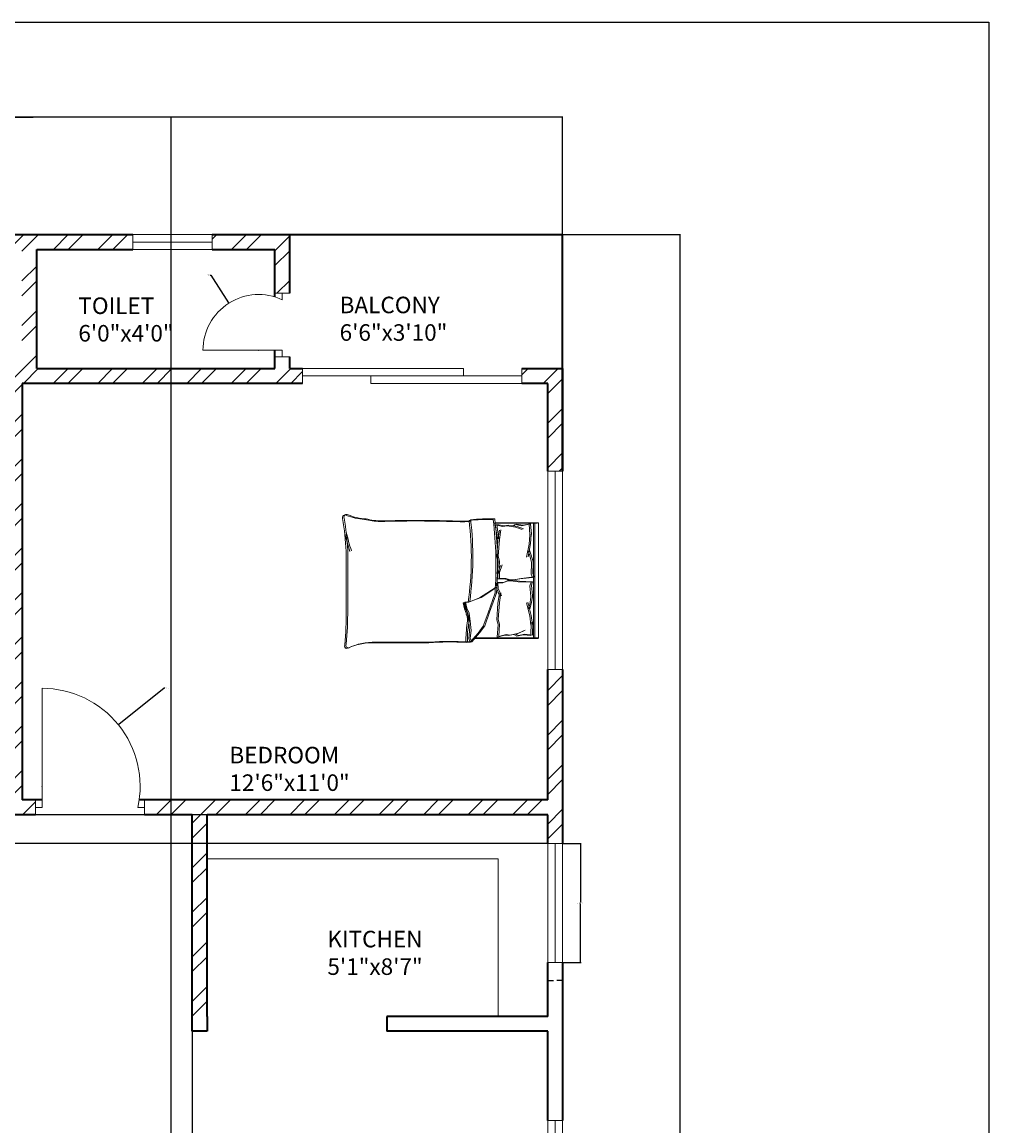
# Model space of a CAD drawing. Units: inches. Extents: x 2064 to 2782, y 1196 to 2299.
# Tile 11 of 11: x 2490 to 2782, y 1965 to 2299. Entities that reach past the tile are written whole.
import ezdxf

# ---------------------------------------------------------------- set-up
doc = ezdxf.new("R2010")
doc.units = ezdxf.units.IN
for name, color, linetype, lineweight in [('A-ANNO-DIMS', 2, 'Continuous', 18), ('A-ANNO-TTLB', 7, 'Continuous', 25), ('A-AREA-IDEN', 7, 'Continuous', 18), ('A-DOOR', 11, 'Continuous', 18), ('A-FLOR-CASE', 8, 'Continuous', 18), ('A-FURN', 8, 'Continuous', 13), ('A-GLAZ', 151, 'Continuous', 18), ('A-WALL', 7, 'Continuous', 35), ('A-WALL-PATT', 9, 'Continuous', 13)]:
    doc.layers.add(name, color=color, linetype=linetype, lineweight=lineweight)
doc.styles.get("Standard").update_dxf_attribs({"font": 'arial.ttf'})
doc.dimstyles.get("Standard").update_dxf_attribs({"dimtxt": 0.18, "dimasz": 0.18, "dimexe": 0.18, "dimexo": 0.0625, "dimgap": 0.09, "dimtad": 0, "dimtih": 1, "dimtoh": 1, "dimdec": 4, "dimzin": 0, "dimdsep": 46, "dimtxsty": 'Standard', "dimcen": 0.09, "dimadec": 0, "dimazin": 0, "dimtfac": 1, "dimtdec": 4, "dimtofl": 0, "dimtmove": 0, "dimatfit": 3, "dimfxl": 1, "dimtolj": 1, "dimtzin": 0, "dimarcsym": 0})

# ---------------------------------------------------------------- blocks, each defined once
blk = doc.blocks.new('BED-DOUBLE')
for p, q in [((2.53, 46.14), (2.53, 59.33)), ((2.53, 46.14), (2.53, 59.33)), ((2.53, 59.33), (37.35, 59.33)), ((2.53, 58.22), (37.35, 58.22)), ((2.53, 58.22), (37.35, 58.22)), ((2.7, 45.67), (2.7, 58.87)), ((2.7, 45.67), (2.7, 58.87)), ((2.7, 57.75), (37.52, 57.75)), ((2.7, 57.75), (37.52, 57.75)), ((2.84, 56.9), (5.96, 57.14)), ((2.84, 56.9), (5.96, 57.14)), ((2.84, 56.92), (3.26, 54.6)), ((2.84, 56.92), (3.26, 54.6)), ((5.96, 57.14), (6.04, 57.13)), ((5.96, 57.14), (6.04, 57.13)), ((6.04, 57.13), (8.82, 56.92)), ((6.04, 57.13), (8.82, 56.92)), ((8.82, 56.92), (12.82, 56.18)), ((8.82, 56.92), (12.82, 56.18)), ((10.82, 56.6), (12.3, 57.13)), ((10.82, 56.6), (12.3, 57.13)), ((12.3, 57.13), (14.4, 57.66)), ((12.3, 57.13), (14.4, 57.66)), ((12.46, 56.66), (14.57, 57.19)), ((12.46, 56.66), (14.57, 57.19)), ((14.4, 57.66), (14.64, 57.66)), ((14.4, 57.66), (14.64, 57.66)), ((14.57, 57.19), (14.8, 57.19)), ((14.57, 57.19), (14.8, 57.19)), ((14.64, 57.66), (17.88, 57.55)), ((14.64, 57.66), (17.88, 57.55)), ((14.8, 57.19), (18.04, 57.09)), ((14.8, 57.19), (18.04, 57.09)), ((17.88, 57.55), (18.93, 57.97)), ((17.88, 57.55), (18.93, 57.97)), ((18.04, 57.09), (19.1, 57.51)), ((18.04, 57.09), (19.1, 57.51)), ((18.93, 57.97), (19.35, 54.07)), ((18.93, 57.97), (19.35, 54.07)), ((19.1, 57.51), (19.52, 53.61)), ((19.1, 57.51), (19.52, 53.61)), ((20.38, 57.52), (20.2, 53.6)), ((20.38, 57.52), (20.21, 53.6)), ((20.55, 57.05), (20.37, 53.14)), ((20.55, 57.05), (20.37, 53.14)), ((21.46, 57.16), (20.38, 57.52)), ((21.46, 57.16), (20.38, 57.52)), ((21.63, 56.7), (20.55, 57.05)), ((21.63, 56.7), (20.55, 57.05)), ((24.69, 57.47), (21.46, 57.16)), ((24.69, 57.47), (21.46, 57.16)), ((24.85, 57.01), (21.63, 56.7)), ((24.85, 57.01), (21.63, 56.7)), ((24.92, 57.49), (24.69, 57.47)), ((24.92, 57.49), (24.69, 57.47)), ((25.09, 57.02), (24.85, 57.01)), ((25.09, 57.02), (24.85, 57.01)), ((27.05, 57.09), (24.92, 57.49)), ((27.05, 57.09), (24.92, 57.49)), ((27.22, 56.63), (25.09, 57.02)), ((27.22, 56.63), (25.09, 57.02)), ((30.54, 57.1), (26.59, 56.11)), ((30.54, 57.1), (26.59, 56.11)), ((28.56, 56.66), (27.05, 57.09)), ((28.56, 56.66), (27.05, 57.09)), ((33.3, 57.48), (30.54, 57.1)), ((33.3, 57.48), (30.54, 57.1)), ((33.47, 57.02), (30.7, 56.63)), ((33.47, 57.02), (30.7, 56.63)), ((36.51, 57.47), (32.57, 57.54)), ((32.57, 57.54), (33.3, 57.48)), ((36.51, 57.47), (32.57, 57.54)), ((32.57, 57.54), (33.3, 57.48)), ((36.68, 57.01), (32.74, 57.08)), ((32.74, 57.08), (33.47, 57.02)), ((36.67, 57.01), (32.74, 57.08)), ((32.74, 57.08), (33.47, 57.02)), ((36.51, 57.47), (36.23, 55.13)), ((36.51, 57.47), (36.23, 55.13)), ((36.68, 57.01), (36.4, 54.67)), ((36.67, 57.01), (36.4, 54.67)), ((37.35, 59.33), (37.35, 39.95)), ((37.35, 59.33), (37.35, 39.95)), ((37.52, 59.33), (37.52, 58.87)), ((37.52, 58.87), (37.52, 39.48)), ((37.52, 58.87), (37.52, 39.48)), ((3.26, 54.6), (2.94, 52.71)), ((3.26, 54.6), (2.94, 52.71)), ((3, 56.45), (3.43, 54.14)), ((3, 56.45), (3.43, 54.14)), ((3.01, 56.44), (6.13, 56.68)), ((3.01, 56.44), (6.13, 56.68)), ((3.43, 54.14), (3.11, 52.24)), ((3.43, 54.14), (3.11, 52.24)), ((3.68, 52.81), (4.42, 54.81)), ((3.68, 52.81), (4.42, 54.81)), ((3.85, 52.34), (4.58, 54.35)), ((3.85, 52.34), (4.58, 54.35)), ((6.13, 56.68), (6.2, 56.66)), ((6.13, 56.68), (6.2, 56.66)), ((6.2, 56.66), (8.99, 56.45)), ((6.2, 56.66), (8.99, 56.45)), ((8.99, 56.45), (12.99, 55.72)), ((8.99, 56.45), (12.99, 55.72)), ((10.99, 56.14), (12.46, 56.66)), ((10.99, 56.14), (12.46, 56.66)), ((19.35, 54.07), (19.77, 51.76)), ((19.35, 54.07), (19.77, 51.76)), ((19.52, 53.61), (19.94, 51.29)), ((19.52, 53.61), (19.94, 51.29)), ((20.21, 53.6), (19.93, 51.26)), ((20.2, 53.6), (19.93, 51.26)), ((30.7, 56.63), (26.75, 55.65)), ((30.7, 56.63), (26.75, 55.65)), ((28.73, 56.19), (27.22, 56.63)), ((28.73, 56.19), (27.22, 56.63)), ((35.92, 53.32), (35.06, 55.27)), ((35.92, 53.32), (35.06, 55.27)), ((36.09, 52.85), (35.23, 54.8)), ((36.09, 52.85), (35.23, 54.8)), ((36.23, 55.13), (36.67, 53.26)), ((36.23, 55.13), (36.67, 53.26)), ((36.4, 54.67), (36.83, 52.79)), ((36.4, 54.67), (36.83, 52.79)), ((2.94, 52.71), (3.36, 51.97)), ((2.94, 52.71), (3.36, 51.97)), ((3.11, 52.24), (3.53, 51.5)), ((3.11, 52.24), (3.53, 51.5)), ((3.26, 50.18), (3.68, 52.81)), ((3.26, 50.18), (3.68, 52.81)), ((3.47, 49.02), (3.26, 50.18)), ((3.47, 49.02), (3.26, 50.18)), ((3.43, 49.71), (3.85, 52.34)), ((3.43, 49.71), (3.85, 52.34)), ((19.77, 50.81), (19.35, 49.44)), ((19.77, 50.81), (19.35, 49.44)), ((19.94, 50.34), (19.52, 48.97)), ((19.94, 50.34), (19.52, 48.97)), ((19.77, 51.76), (19.77, 50.81)), ((19.77, 51.76), (19.77, 50.81)), ((19.93, 51.26), (19.99, 50.32)), ((19.93, 51.26), (19.99, 50.32)), ((19.94, 51.29), (19.94, 50.34)), ((19.94, 51.29), (19.94, 50.34)), ((19.99, 50.32), (20.49, 48.98)), ((19.99, 50.32), (20.49, 48.98)), ((20.37, 53.14), (20.1, 50.8)), ((20.37, 53.14), (20.1, 50.8)), ((20.1, 50.8), (20.15, 49.85)), ((20.1, 50.8), (20.15, 49.85)), ((36.51, 50.72), (35.92, 53.32)), ((36.51, 50.72), (35.92, 53.32)), ((36.68, 50.25), (36.09, 52.85)), ((36.67, 50.25), (36.09, 52.85)), ((36.67, 53.26), (36.29, 52.5)), ((36.67, 53.26), (36.29, 52.5)), ((36.37, 49.55), (36.51, 50.72)), ((36.37, 49.55), (36.51, 50.72)), ((36.83, 52.79), (36.46, 52.03)), ((36.83, 52.79), (36.46, 52.03)), ((36.54, 49.08), (36.68, 50.25)), ((36.54, 49.08), (36.67, 50.25)), ((3.05, 46.7), (3.47, 49.02)), ((3.05, 46.7), (3.47, 49.02)), ((6.76, 47.23), (3.05, 46.7)), ((6.76, 47.23), (3.05, 46.7)), ((3.21, 46.24), (3.64, 48.55)), ((3.21, 46.24), (3.64, 48.55)), ((6.93, 46.76), (3.21, 46.24)), ((6.93, 46.76), (3.21, 46.24)), ((3.64, 48.55), (3.43, 49.71)), ((3.64, 48.55), (3.43, 49.71)), ((4.65, 47.95), (7.59, 47.46)), ((4.65, 47.95), (7.59, 47.46)), ((4.82, 47.48), (7.75, 47)), ((4.82, 47.48), (7.75, 47)), ((7.59, 47.46), (6.76, 47.23)), ((7.59, 47.46), (6.76, 47.23)), ((7.75, 47), (6.93, 46.76)), ((7.75, 47), (6.93, 46.76)), ((7.59, 47.46), (12.69, 47.15)), ((7.59, 47.46), (12.69, 47.15)), ((7.75, 47), (12.86, 46.68)), ((7.75, 47), (12.86, 46.68)), ((12.69, 47.15), (14.12, 47.55)), ((12.69, 47.15), (14.12, 47.55)), ((12.86, 46.68), (14.29, 47.09)), ((12.86, 46.68), (14.29, 47.09)), ((14.12, 47.55), (17.86, 47.26)), ((14.12, 47.55), (17.86, 47.26)), ((14.29, 47.09), (18.03, 46.79)), ((14.29, 47.09), (18.03, 46.79)), ((17.56, 47.49), (15.27, 48.28)), ((17.56, 47.49), (15.27, 48.28)), ((17.73, 47.02), (15.44, 47.82)), ((17.73, 47.02), (15.44, 47.82)), ((19.35, 47.49), (17.56, 47.49)), ((19.35, 47.49), (17.56, 47.49)), ((19.52, 47.02), (17.73, 47.02)), ((19.52, 47.02), (17.73, 47.02)), ((19.35, 49.44), (19.35, 47.49)), ((19.35, 49.44), (19.35, 47.49)), ((19.52, 48.97), (19.52, 47.02)), ((19.52, 48.97), (19.52, 47.02)), ((20.15, 49.85), (20.66, 48.51)), ((20.15, 49.85), (20.66, 48.51)), ((20.49, 48.98), (20.62, 47.03)), ((20.49, 48.98), (20.62, 47.03)), ((20.62, 47.03), (22.4, 47.14)), ((20.62, 47.03), (22.4, 47.14)), ((20.66, 48.51), (20.78, 46.56)), ((20.66, 48.51), (20.78, 46.56)), ((22.4, 47.14), (24.64, 48.08)), ((22.4, 47.14), (24.64, 48.08)), ((22.57, 46.67), (24.81, 47.61)), ((22.57, 46.67), (24.81, 47.61)), ((23.72, 47.95), (26.66, 47.46)), ((23.72, 47.95), (26.66, 47.46)), ((23.89, 47.48), (26.83, 47)), ((23.89, 47.48), (26.83, 47)), ((26.66, 47.46), (31.77, 47.15)), ((26.66, 47.46), (31.77, 47.15)), ((26.83, 47), (31.94, 46.68)), ((26.83, 47), (31.94, 46.68)), ((31.77, 47.15), (33.2, 47.55)), ((31.77, 47.15), (33.2, 47.55)), ((31.94, 46.68), (33.36, 47.09)), ((31.94, 46.68), (33.36, 47.09)), ((33.2, 47.55), (36.94, 47.26)), ((33.2, 47.55), (36.94, 47.26)), ((33.36, 47.09), (37.1, 46.79)), ((33.36, 47.09), (37.1, 46.79)), ((36.94, 47.26), (36.37, 49.55)), ((36.94, 47.26), (36.37, 49.55)), ((37.1, 46.79), (36.54, 49.08)), ((37.1, 46.79), (36.54, 49.08)), ((20.78, 46.56), (22.57, 46.67)), ((20.78, 46.56), (22.57, 46.67)), ((22.05, 46.67), (25.1, 41.94)), ((22.05, 46.67), (25.1, 41.94)), ((22.21, 46.2), (25.26, 41.47)), ((22.21, 46.2), (25.26, 41.47)), ((29.61, 44.53), (23.54, 46.67)), ((29.61, 44.53), (23.54, 46.67)), ((29.78, 44.07), (23.7, 46.2)), ((29.78, 44.07), (23.7, 46.2)), ((33.67, 43.07), (29.61, 44.53)), ((33.67, 43.07), (29.61, 44.53)), ((33.84, 42.6), (29.78, 44.07)), ((33.84, 42.6), (29.78, 44.07)), ((25.1, 41.94), (26.34, 38.67)), ((25.1, 41.94), (26.34, 38.67)), ((25.26, 41.47), (26.51, 38.2)), ((25.26, 41.47), (26.51, 38.2)), ((35.82, 41.49), (33.67, 43.07)), ((35.82, 41.49), (33.67, 43.07)), ((35.98, 41.02), (33.84, 42.6)), ((35.98, 41.02), (33.84, 42.6)), ((38.52, 39.12), (35.82, 41.49)), ((38.52, 39.12), (35.82, 41.49)), ((38.68, 38.65), (35.98, 41.02)), ((38.68, 38.65), (35.98, 41.02)), ((26.34, 38.67), (26.56, 37.2)), ((26.34, 38.67), (26.56, 37.2)), ((26.51, 38.2), (26.73, 36.74)), ((26.51, 38.2), (26.73, 36.74)), ((26.56, 37.2), (28.37, 37.65)), ((26.56, 37.2), (28.37, 37.65)), ((26.73, 36.74), (28.54, 37.19)), ((26.73, 36.74), (28.54, 37.19)), ((28.37, 37.65), (29.84, 38.33)), ((28.37, 37.65), (29.84, 38.33)), ((28.54, 37.19), (30, 37.87)), ((28.54, 37.19), (30, 37.87)), ((29.84, 38.33), (32.32, 38.67)), ((29.84, 38.33), (32.32, 38.67)), ((30, 37.87), (32.49, 38.2)), ((30, 37.87), (32.49, 38.2)), ((32.32, 38.67), (35.14, 38.9)), ((32.32, 38.67), (35.14, 38.9)), ((32.49, 38.2), (35.31, 38.43)), ((32.49, 38.2), (35.31, 38.43)), ((35.14, 38.9), (37.4, 38.67)), ((35.14, 38.9), (37.4, 38.67)), ((35.31, 38.43), (37.56, 38.2)), ((35.31, 38.43), (37.56, 38.2)), ((37.4, 38.67), (38.52, 39.12)), ((37.4, 38.67), (38.52, 39.12)), ((37.56, 38.2), (38.68, 38.65)), ((37.56, 38.2), (38.68, 38.65)), ((38.57, 37.85), (38.52, 39.12, 2.82)), ((38.57, 37.85), (38.52, 39.12, 2.82)), ((38.74, 37.38), (38.68, 38.65, 2.82)), ((38.74, 37.38), (38.68, 38.65, 2.82)), ((10.97, 1.6), (28.91, 1.6)), ((10.97, 1.6), (28.91, 1.6)), ((11.14, 1.14), (29.07, 1.14)), ((11.14, 1.14), (29.07, 1.14))]:
    blk.add_line(p, q)
for centre, radius, start, end in [((15.56, -73.3), 120.19, 86.0865, 96.7821), ((15.56, -73.3), 120.19, 86.0865, 96.7821), ((62.04, 44.69), 60.69, 178.7218, 185.604), ((62.04, 44.69), 60.69, 178.7218, 185.604), ((62.21, 44.23), 60.69, 178.7218, 185.604), ((62.21, 44.23), 60.69, 178.7218, 185.604), ((15.73, -73.76), 120.19, 86.0865, 96.7821), ((15.73, -73.76), 120.19, 86.0865, 96.7821), ((12.94, -54.55), 94, 81.7845, 96.9006), ((12.94, -54.55), 94, 81.7845, 96.9006), ((13.1, -55.01), 94, 81.7845, 96.9006), ((13.1, -55.01), 94, 81.7845, 96.9006), ((-121.89, 36.62), 123.93, 358.4762, 1.0082), ((-121.89, 36.62), 123.93, 358.4762, 1.0082), ((-121.72, 36.16), 123.93, 358.4762, 1.0082), ((-121.72, 36.16), 123.93, 358.4762, 1.0082), ((26.69, 37.16), 0.134, 160.2464, 271.1377), ((26.69, 37.16), 0.134, 160.2464, 271.1377), ((22.7, 58.25), 21.6, 280.6617, 289.8806), ((22.7, 58.25), 21.6, 280.6617, 289.8806), ((26.86, 36.69), 0.134, 160.2464, 271.1377), ((26.86, 36.69), 0.134, 160.2464, 271.1377), ((22.86, 57.79), 21.6, 280.6617, 289.8806), ((22.86, 57.79), 21.6, 280.6617, 289.8806), ((31.87, 33.79), 4.53, 78.6608, 113.7384), ((31.87, 33.79), 4.53, 78.6608, 113.7384), ((32.04, 33.32), 4.53, 78.6608, 113.7384), ((32.04, 33.32), 4.53, 78.6608, 113.7384), ((37.39, 64.18), 26.36, 259.8763, 272.5657), ((37.39, 64.18), 26.36, 259.8763, 272.5657), ((37.56, 63.72), 26.36, 259.8763, 272.5657), ((37.56, 63.72), 26.36, 259.8763, 272.5657), ((132.79, 32.88), 94.35, 176.9791, 183.8365), ((132.79, 32.88), 94.35, 176.9791, 183.8365), ((132.95, 32.41), 94.35, 176.9791, 183.8365), ((132.95, 32.41), 94.35, 176.9791, 183.8365), ((353.21, 22.46), 351.38, 178.2277, 181.7185), ((353.21, 22.46), 351.38, 178.2277, 181.7185), ((353.38, 21.99), 351.38, 178.2277, 181.7185), ((353.38, 21.99), 351.38, 178.2277, 181.7185), ((-3284.8, 9.92), 3323.5, 0.00217, 0.28689), ((-3284.8, 9.92), 3323.5, 0.00217, 0.28689), ((-3284.64, 9.46), 3323.5, 0.00217, 0.28689), ((-3284.64, 9.46), 3323.5, 0.00217, 0.28689), ((-19.6, 12.33), 21.59, 346.0648, 358.9113), ((-19.6, 12.33), 21.59, 346.0648, 358.9113), ((-19.43, 11.87), 21.59, 346.0648, 358.9113), ((-19.43, 11.87), 21.59, 346.0648, 358.9113), ((55.48, 9.31), 16.8, 177.4714, 206.4681), ((55.48, 9.31), 16.8, 177.4714, 206.4681), ((-15.78, 8.14), 17.17, 337.9751, 356.652), ((-15.78, 8.14), 17.17, 337.9751, 356.652), ((55.65, 8.84), 16.8, 177.4714, 206.4681), ((55.65, 8.84), 16.8, 177.4714, 206.4681), ((-15.61, 7.67), 17.17, 337.9751, 356.652), ((-15.61, 7.67), 17.17, 337.9751, 356.652), ((0.79, 1.26), 0.793, 146.1736, 293.4781), ((0.79, 1.26), 0.793, 146.1736, 293.4781), ((0.96, 0.79), 0.793, 146.1736, 293.4781), ((0.96, 0.79), 0.793, 146.1736, 293.4781), ((15.61, -86.98), 88.71, 92.9958, 99.4091), ((15.61, -86.98), 88.71, 92.9958, 99.4091), ((15.78, -87.45), 88.71, 92.9958, 99.4091), ((15.78, -87.45), 88.71, 92.9958, 99.4091), ((-12.55, 76.61), 77.56, 283.3832, 287.7053), ((-12.55, 76.61), 77.56, 283.3832, 287.7053), ((-12.38, 76.14), 77.56, 283.3832, 287.7053), ((-12.38, 76.14), 77.56, 283.3832, 287.7053), ((29.98, -95.32), 96.92, 84.4998, 90.6351), ((29.98, -95.32), 96.92, 84.4998, 90.6351), ((30.15, -95.78), 96.92, 84.4998, 90.6351), ((30.15, -95.78), 96.92, 84.4998, 90.6351), ((39.64, 1.87), 0.803, 242.6588, 356.02), ((39.64, 1.87), 0.803, 242.6588, 356.02), ((39.81, 1.41), 0.803, 242.6588, 356.02), ((39.81, 1.41), 0.803, 242.6588, 356.02)]:
    blk.add_arc(centre, radius, start, end)
blk = doc.blocks.new('WIN-60IN')
for p, q in [((0, 4.5), (0, 0)), ((60, 4.5), (0, 4.5)), ((60, 2.25), (60, 4.5)), ((60, 4.5), (60, 0)), ((0, 0), (0, 2.25)), ((0, 2.25), (60, 2.25)), ((0, 0), (60, 0))]:
    blk.add_line(p, q)
blk = doc.blocks.new('WIN-36IN')
for p, q in [((0, 36), (4.5, 36)), ((0, 36), (0, 0)), ((4.5, 36), (2.25, 36)), ((2.25, 36), (2.25, 0)), ((4.5, 36), (4.5, 0)), ((2.25, 0), (0, 0)), ((0, 0), (4.5, 0))]:
    blk.add_line(p, q)
blk = doc.blocks.new('WIN-24IN')
for p, q in [((0, 0), (0, 4.5)), ((0, 4.5), (0, 2.25)), ((0, 4.5), (24, 4.5)), ((24, 2.25), (24, 4.5)), ((24, 4.5), (24, 0)), ((0, 2.25), (24, 2.25)), ((24, 0), (0, 0))]:
    blk.add_line(p, q)
blk = doc.blocks.new('*D12')
at = {"layer": 'A-ANNO-DIMS', "color": 0, "lineweight": -2, "transparency": 16777216}
for p, q in [((2653.23, 2050.11), (2658.75, 2050.11)), ((2658.57, 2049.93), (2658.57, 2032.29)), ((2658.57, 2014.29), (2658.57, 2031.93)), ((2653.23, 2014.11), (2658.75, 2014.11))]:
    blk.add_line(p, q, dxfattribs=at)
at = {"layer": 'A-ANNO-DIMS', "color": 0, "transparency": 16777216}
for points in [[(2658.54, 2049.93), (2658.6, 2049.93), (2658.57, 2050.11)], [(2658.54, 2014.29), (2658.6, 2014.29), (2658.57, 2014.11)]]:
    blk.add_solid(points, dxfattribs=at)
at = {"layer": 'Defpoints', "color": 0, "transparency": 16777216}
for p in [(2653.17, 2050.11), (2658.57, 2050.11), (2653.17, 2014.11)]:
    blk.add_point(p, dxfattribs=at)
at = {"layer": 'A-ANNO-DIMS', "color": 0, "transparency": 16777216, "insert": (2658.57, 2032.11), "char_height": 0.18, "attachment_point": 5}
blk.add_mtext('\\A1;WINDOW 36 TYP.', dxfattribs=at)
blk = doc.blocks.new('*D13')
at = {"layer": 'A-ANNO-DIMS', "color": 0, "lineweight": -2, "transparency": 16777216}
for p, q in [((2648.67, 2014.05), (2648.67, 2008.53)), ((2653.17, 2014.05), (2653.17, 2008.53)), ((2648.85, 2008.71), (2650.46, 2008.71)), ((2652.99, 2008.71), (2651.38, 2008.71))]:
    blk.add_line(p, q, dxfattribs=at)
at = {"layer": 'A-ANNO-DIMS', "color": 0, "transparency": 16777216}
for points in [[(2648.85, 2008.74), (2648.85, 2008.68), (2648.67, 2008.71)], [(2652.99, 2008.74), (2652.99, 2008.68), (2653.17, 2008.71)]]:
    blk.add_solid(points, dxfattribs=at)
at = {"layer": 'Defpoints', "color": 0, "transparency": 16777216}
for p in [(2648.67, 2014.11), (2653.17, 2014.11), (2653.17, 2008.71)]:
    blk.add_point(p, dxfattribs=at)
at = {"layer": 'A-ANNO-DIMS', "color": 0, "transparency": 16777216, "insert": (2650.92, 2008.71), "char_height": 0.18, "attachment_point": 5}
blk.add_mtext('\\A1;5 TYP.', dxfattribs=at)
blk = doc.blocks.new('*D22')
at = {"layer": 'A-ANNO-DIMS', "color": 0, "lineweight": -2, "transparency": 16777216}
for p, q in [((2128.17, 2234.35), (2128.17, 2269.97)), ((2128.35, 2269.79), (2390.38, 2269.79)), ((2652.99, 2269.79), (2390.96, 2269.79)), ((2653.17, 2234.35), (2653.17, 2269.97))]:
    blk.add_line(p, q, dxfattribs=at)
at = {"layer": 'A-ANNO-DIMS', "color": 0, "transparency": 16777216}
for points in [[(2128.35, 2269.82), (2128.35, 2269.76), (2128.17, 2269.79)], [(2652.99, 2269.82), (2652.99, 2269.76), (2653.17, 2269.79)]]:
    blk.add_solid(points, dxfattribs=at)
at = {"layer": 'Defpoints', "color": 0, "transparency": 16777216}
for p in [(2653.17, 2269.79), (2128.17, 2234.29), (2653.17, 2234.29)]:
    blk.add_point(p, dxfattribs=at)
at = {"layer": 'A-ANNO-DIMS', "color": 0, "transparency": 16777216, "insert": (2390.67, 2269.79), "char_height": 0.18, "attachment_point": 5}
blk.add_mtext('\\A1;525', dxfattribs=at)
blk = doc.blocks.new('*D23')
at = {"layer": 'A-ANNO-DIMS', "color": 0, "lineweight": -2, "transparency": 16777216}
for p, q in [((2653.23, 2234.29), (2688.85, 2234.29)), ((2688.67, 2234.11), (2688.67, 1937.72)), ((2688.67, 1640.97), (2688.67, 1937.36)), ((2452.23, 1640.79), (2688.85, 1640.79))]:
    blk.add_line(p, q, dxfattribs=at)
at = {"layer": 'A-ANNO-DIMS', "color": 0, "transparency": 16777216}
for points in [[(2688.64, 2234.11), (2688.7, 2234.11), (2688.67, 2234.29)], [(2688.64, 1640.97), (2688.7, 1640.97), (2688.67, 1640.79)]]:
    blk.add_solid(points, dxfattribs=at)
at = {"layer": 'Defpoints', "color": 0, "transparency": 16777216}
for p in [(2653.17, 2234.29), (2688.67, 2234.29), (2452.17, 1640.79)]:
    blk.add_point(p, dxfattribs=at)
at = {"layer": 'A-ANNO-DIMS', "color": 0, "transparency": 16777216, "insert": (2688.67, 1937.54), "char_height": 0.18, "attachment_point": 5}
blk.add_mtext('\\A1;593.5', dxfattribs=at)
blk = doc.blocks.new('*D27')
at = {"layer": 'A-ANNO-DIMS', "color": 0, "lineweight": -2, "transparency": 16777216}
for p, q in [((2452.17, 1640.85), (2452.17, 2269.97)), ((2452.35, 2269.79), (2493.09, 2269.79)), ((2534.61, 2269.79), (2493.87, 2269.79)), ((2534.79, 1643.35), (2534.79, 2269.97))]:
    blk.add_line(p, q, dxfattribs=at)
at = {"layer": 'A-ANNO-DIMS', "color": 0, "transparency": 16777216}
for points in [[(2452.35, 2269.82), (2452.35, 2269.76), (2452.17, 2269.79)], [(2534.61, 2269.82), (2534.61, 2269.76), (2534.79, 2269.79)]]:
    blk.add_solid(points, dxfattribs=at)
at = {"layer": 'Defpoints', "color": 0, "transparency": 16777216}
for p in [(2534.79, 2269.79), (2534.79, 1643.29), (2452.17, 1640.79)]:
    blk.add_point(p, dxfattribs=at)
at = {"layer": 'A-ANNO-DIMS', "color": 0, "transparency": 16777216, "insert": (2493.48, 2269.79), "char_height": 0.18, "attachment_point": 5}
blk.add_mtext('\\A1;82.62', dxfattribs=at)
blk = doc.blocks.new('*D36')
at = {"layer": 'A-ANNO-DIMS', "color": 0, "lineweight": -2, "transparency": 16777216}
for p, q in [((2390.62, 2058.73), (2390.62, 1539.01)), ((2541.17, 2058.73), (2541.17, 1539.01)), ((2390.8, 1539.19), (2465.44, 1539.19)), ((2540.99, 1539.19), (2466.35, 1539.19))]:
    blk.add_line(p, q, dxfattribs=at)
at = {"layer": 'A-ANNO-DIMS', "color": 0, "transparency": 16777216}
for points in [[(2390.8, 1539.22), (2390.8, 1539.16), (2390.62, 1539.19)], [(2540.99, 1539.22), (2540.99, 1539.16), (2541.17, 1539.19)]]:
    blk.add_solid(points, dxfattribs=at)
at = {"layer": 'Defpoints', "color": 0, "transparency": 16777216}
for p in [(2390.62, 2058.79), (2541.17, 2058.79), (2541.17, 1539.19)]:
    blk.add_point(p, dxfattribs=at)
at = {"layer": 'A-ANNO-DIMS', "color": 0, "transparency": 16777216, "insert": (2465.9, 1539.19), "char_height": 0.18, "attachment_point": 5}
blk.add_mtext('\\A1;150.55', dxfattribs=at)
blk = doc.blocks.new('*D40')
at = {"layer": 'A-ANNO-DIMS', "color": 0, "lineweight": -2, "transparency": 16777216}
for p, q in [((2648.61, 2058.79), (2092.49, 2058.79)), ((2092.67, 2058.61), (2092.67, 2054.63)), ((2092.67, 2050.29), (2092.67, 2054.27)), ((2648.61, 2050.11), (2092.49, 2050.11))]:
    blk.add_line(p, q, dxfattribs=at)
at = {"layer": 'A-ANNO-DIMS', "color": 0, "transparency": 16777216}
for points in [[(2092.64, 2058.61), (2092.7, 2058.61), (2092.67, 2058.79)], [(2092.64, 2050.29), (2092.7, 2050.29), (2092.67, 2050.11)]]:
    blk.add_solid(points, dxfattribs=at)
at = {"layer": 'Defpoints', "color": 0, "transparency": 16777216}
for p in [(2092.67, 2058.79), (2648.67, 2058.79), (2648.67, 2050.11)]:
    blk.add_point(p, dxfattribs=at)
at = {"layer": 'A-ANNO-DIMS', "color": 0, "transparency": 16777216, "insert": (2092.67, 2054.45), "char_height": 0.18, "attachment_point": 5}
blk.add_mtext('\\A1;8.682', dxfattribs=at)
blk = doc.blocks.new('*D44')
at = {"layer": 'A-ANNO-DIMS', "color": 0, "lineweight": -2, "transparency": 16777216}
for p, q in [((2532.73, 2097.13), (2519.01, 2086.09)), ((2532.91, 2097.13), (2532.73, 2097.13)), ((2495.67, 2067.39), (2495.85, 2067.39)), ((2495.76, 2067.3), (2495.76, 2067.48))]:
    blk.add_line(p, q, dxfattribs=at)
at = {"layer": 'A-ANNO-DIMS', "color": 0, "transparency": 16777216}
blk.add_solid([(2518.99, 2086.11), (2519.02, 2086.07), (2518.86, 2085.98)], dxfattribs=at)
at = {"layer": 'Defpoints', "color": 0, "transparency": 16777216}
for p in [(2518.86, 2085.98), (2495.76, 2067.39)]:
    blk.add_point(p, dxfattribs=at)
at = {"layer": 'A-ANNO-DIMS', "color": 0, "transparency": 16777216, "insert": (2533.46, 2097.13), "char_height": 0.18, "attachment_point": 5}
blk.add_mtext('\\A1;R29.653', dxfattribs=at)
blk = doc.blocks.new('*D52')
at = {"layer": 'A-ANNO-DIMS', "color": 0, "lineweight": -2, "transparency": 16777216}
for p, q in [((2546.63, 2222.06), (2546.81, 2222.06)), ((2546.81, 2222.06), (2552.13, 2213.68)), ((2561.18, 2199.31), (2561.36, 2199.31)), ((2561.27, 2199.22), (2561.27, 2199.4))]:
    blk.add_line(p, q, dxfattribs=at)
at = {"layer": 'A-ANNO-DIMS', "color": 0, "transparency": 16777216}
blk.add_solid([(2552.16, 2213.69), (2552.11, 2213.66), (2552.23, 2213.52)], dxfattribs=at)
at = {"layer": 'Defpoints', "color": 0, "transparency": 16777216}
for p in [(2552.23, 2213.52), (2561.27, 2199.31)]:
    blk.add_point(p, dxfattribs=at)
at = {"layer": 'A-ANNO-DIMS', "color": 0, "transparency": 16777216, "insert": (2546.15, 2222.06), "char_height": 0.18, "attachment_point": 5}
blk.add_mtext('\\A1;R16.85', dxfattribs=at)

msp = doc.modelspace()

# ---------------------------------------------------------------- hatches: boundary and pattern name
at = {"layer": 'A-WALL-PATT'}
h = msp.add_hatch(dxfattribs=at)
h.set_pattern_fill('ANSI32', color=256)
h.paths.add_polyline_path([(2489.7688, 2189.2917), (2574.5454, 2189.2917), (2574.5454, 2191.5417), (2574.5454, 2193.7917), (2570.6691, 2193.7917), (2570.6691, 2197.3052), (2568.4191, 2197.3052), (2566.1691, 2197.3052), (2566.1691, 2193.7917), (2494.1691, 2193.7917), (2494.1691, 2229.7917), (2523.2441, 2229.7917), (2523.2441, 2234.2917), (2471.2886, 2234.2917), (2471.2886, 2229.7917), (2489.6691, 2229.7917), (2489.6691, 2193.7917), (2417.6691, 2193.7917), (2417.6691, 2197.0632), (2415.4191, 2197.0632), (2413.1691, 2197.0632), (2413.1691, 2193.7917), (2406.8865, 2193.7917), (2406.8865, 2189.2917), (2485.2688, 2189.2917), (2485.2688, 2063.2917), (2369.1629, 2063.2917), (2369.1629, 2058.7917), (2386.1222, 2058.7917), (2386.1222, 1856.2917), (2382.1576, 1856.2917), (2382.1576, 1851.7917), (2394.9764, 1851.7917), (2394.9764, 1854.0417), (2394.9764, 1856.2917), (2390.6222, 1856.2917), (2390.6222, 2058.7917), (2485.2688, 2058.7917), (2493.762, 2058.7917), (2493.762, 2061.0417), (2493.762, 2063.2917), (2489.7688, 2063.2917)])
h.paths.add_polyline_path([(2447.2886, 2234.2917), (2413.1691, 2234.2917), (2413.1691, 2217.3799), (2417.6691, 2217.3799), (2417.6691, 2229.7917), (2447.2886, 2229.7917)], flags=17)
h.paths.add_polyline_path([(2570.6691, 2234.2917), (2547.2441, 2234.2917), (2547.2441, 2229.7917), (2566.1691, 2229.7917), (2566.1691, 2216.5615), (2570.6691, 2216.5615)], flags=17)
h.paths.add_polyline_path([(2653.1691, 2189.2917), (2653.1691, 2193.7917), (2640.8843, 2193.7917), (2640.8843, 2189.2917), (2648.6691, 2189.2917), (2648.6691, 2162.7138), (2653.1691, 2162.7138)])
h.paths.add_polyline_path([(2653.1691, 2102.7138), (2648.6691, 2102.7138), (2648.6691, 2063.2917), (2526.7281, 2063.2917), (2526.7281, 2058.7917), (2541.1691, 2058.7917), (2541.1691, 1993.2917), (2545.6691, 1993.2917), (2545.6691, 1997.7917), (2545.6691, 2058.7917), (2648.6691, 2058.7917), (2648.6691, 2050.1099), (2653.1691, 2050.1099)])
h.paths.add_polyline_path([(2600.6691, 1856.2917), (2493.4607, 1856.2917), (2493.4607, 1851.7917), (2596.1691, 1851.7917), (2596.1691, 1695.7917), (2594.0816, 1695.7917), (2594.0816, 1691.2917), (2614.7905, 1691.2917), (2614.7905, 1645.2917), (2536.7905, 1645.2917), (2536.7905, 1691.2917), (2539.332, 1691.2917), (2539.332, 1693.5417), (2539.332, 1695.7917), (2452.1691, 1695.7917), (2452.1691, 1851.7917), (2456.0775, 1851.7917), (2456.0775, 1856.2917), (2427.1536, 1856.2917), (2427.1536, 1851.7917), (2447.6691, 1851.7917), (2447.6691, 1695.7917), (2447.6691, 1645.2917), (2405.1469, 1645.2917), (2405.1469, 1640.7917), (2452.1691, 1640.7917), (2452.1691, 1645.2917), (2452.1691, 1691.2917), (2534.7905, 1691.2917), (2534.7905, 1645.2917), (2534.7905, 1643.2917), (2614.7905, 1643.2917), (2616.7905, 1643.2917), (2616.7905, 1691.2917), (2622.4029, 1691.2917), (2622.4029, 1693.7143), (2622.4029, 1695.7917), (2600.6691, 1695.7917), (2600.6691, 1779.7917), (2648.6691, 1779.7917), (2648.6691, 1695.7917), (2646.4029, 1695.7917), (2646.4029, 1691.2917), (2653.1691, 1691.2917), (2653.1691, 1906.3508), (2648.6691, 1906.3508), (2648.6691, 1856.2917), (2648.6691, 1784.2917), (2600.6691, 1784.2917)])
h.paths.add_polyline_path([(2322.9532, 1819.5181), (2320.7032, 1819.5181), (2318.4532, 1819.5181), (2318.4532, 1695.7917), (2242.7664, 1695.7917), (2242.7664, 1691.2917), (2318.4532, 1691.2917), (2318.4532, 1640.7917), (2322.9532, 1640.7917), (2345.1469, 1640.7917), (2345.1469, 1643.0417), (2345.1469, 1645.2917), (2322.9532, 1645.2917), (2322.9532, 1691.2917), (2322.9532, 1695.7917)])
h.paths.add_polyline_path([(2166.1825, 1691.2917), (2164.1825, 1691.2917), (2164.1825, 1643.2917), (2166.1825, 1643.2917), (2246.1825, 1643.2917), (2246.1825, 1645.2917), (2246.1825, 1691.2917), (2244.1825, 1691.2917), (2244.1825, 1645.2917), (2166.1825, 1645.2917)])
h.paths.add_polyline_path([(2309.404, 1932.7917), (2204.1691, 1932.7917), (2204.1691, 1960.0962), (2199.6691, 1960.0962), (2199.6691, 1932.7917), (2132.6691, 1932.7917), (2132.6691, 1951.0737), (2128.1691, 1951.0737), (2128.1691, 1910.0412), (2132.6691, 1910.0412), (2132.6691, 1928.2917), (2304.904, 1928.2917), (2304.904, 1856.2917), (2304.904, 1851.7917), (2318.4532, 1851.7917), (2318.4532, 1848.8308), (2322.9532, 1848.8308), (2322.9532, 1851.7917), (2347.7631, 1851.7917), (2347.7631, 1856.2917), (2309.404, 1856.2917)])
h.paths.add_polyline_path([(2132.6691, 2044.9092), (2130.4191, 2044.9092), (2128.1691, 2044.9092), (2128.1691, 1987.0737), (2132.6691, 1987.0737), (2132.6691, 2004.7917), (2199.6691, 2004.7917), (2204.1691, 2004.7917), (2204.1691, 2009.2917), (2132.6691, 2009.2917)])
h.paths.add_polyline_path([(2186.6691, 2195.9329), (2184.4191, 2195.9329), (2184.4191, 2195.8929), (2182.1691, 2195.9329), (2182.1691, 2193.7917), (2128.1691, 2193.7917), (2128.1691, 2181.4967), (2132.6691, 2181.4967), (2132.6691, 2182.7769), (2132.6691, 2189.2917), (2182.1691, 2189.2917), (2182.1691, 2135.2917), (2179.804, 2135.2917), (2179.804, 2130.7917), (2190.215, 2130.7917), (2190.215, 2133.0417), (2190.215, 2135.2917), (2186.6691, 2135.2917)])
h.paths.add_polyline_path([(2340.0628, 2189.2917), (2340.0628, 2191.5417), (2340.0628, 2193.7917), (2335.1691, 2193.7917), (2335.1691, 2234.2917), (2280.6746, 2234.2917), (2280.6746, 2229.7917), (2330.6691, 2229.7917), (2330.6691, 2193.7917), (2330.6691, 2135.2917), (2218.6309, 2135.2917), (2218.6309, 2130.7917), (2330.7688, 2130.7917), (2330.7688, 2008.4023), (2335.2688, 2008.4023), (2335.2688, 2058.7917), (2338.9208, 2058.7917), (2338.9208, 2061.0417), (2338.9208, 2063.2917), (2335.2688, 2063.2917), (2335.2688, 2189.2917)])
h.paths.add_polyline_path([(2220.6746, 2234.2917), (2182.1691, 2234.2917), (2182.1691, 2227.4187), (2186.6691, 2227.4187), (2186.6691, 2229.7917), (2220.6746, 2229.7917), (2220.6746, 2232.0417)])
h.paths.add_polyline_path([(2158.8146, 2135.2917), (2132.6691, 2135.2917), (2132.6691, 2157.4967), (2128.1691, 2157.4967), (2128.1691, 2104.9092), (2132.6691, 2104.9092), (2132.6691, 2130.7917), (2158.8146, 2130.7917), (2158.8146, 2133.0417)])
h.paths.add_polyline_path([(2396.0464, 2062.2045), (2434.8868, 2062.2045), (2434.8868, 2080.8619), (2396.0464, 2080.8619)], flags=24)
h.paths.add_polyline_path([(2196.1396, 1653.3449), (2232.023, 1653.3449), (2232.023, 1672.0022), (2196.1396, 1672.0022)], flags=25)

# ---------------------------------------------------------------- linework, layer by layer
at = {"layer": 'A-ANNO-TTLB'}
msp.add_lwpolyline([(2063.9994, 2298.574), (2782.0941, 2298.574), (2782.0941, 1490.6238), (2063.9994, 1490.6238)], close=True, dxfattribs=at)
at = {"layer": 'A-DOOR'}
for p, q in [((2566.1691, 2216.5615), (2570.6691, 2216.5615)), ((2570.6691, 2216.5615), (2568.4191, 2216.5615)), ((2568.4191, 2216.5615), (2568.4191, 2214.5615)), ((2568.4191, 2199.3052), (2544.4191, 2199.3052)), ((2566.1691, 2197.3052), (2570.6691, 2197.3052)), ((2568.4191, 2197.3052), (2568.4191, 2199.3052)), ((2570.6691, 2197.3052), (2568.4191, 2197.3052)), ((2495.762, 2061.0417), (2495.762, 2097.0417)), ((2493.762, 2063.2917), (2493.762, 2058.7917)), ((2493.762, 2058.7917), (2493.762, 2061.0417)), ((2493.762, 2061.0417), (2495.762, 2061.0417)), ((2526.7281, 2061.0417), (2524.7281, 2061.0417)), ((2526.7281, 2063.2917), (2526.7281, 2058.7917)), ((2526.7281, 2058.7917), (2526.7281, 2061.0417))]:
    msp.add_line(p, q, dxfattribs=at)
for centre, radius, start, end in [((2561.2681, 2199.3052), 16.8491, 64.886558, 180), ((2495.762, 2067.3884), 29.6533, 347.641315, 90)]:
    msp.add_arc(centre, radius, start, end, dxfattribs=at)
at = {"layer": 'A-FLOR-CASE'}
for p, q in [((2545.6691, 2045.483), (2633.7392, 2045.483)), ((2633.7392, 2045.483), (2633.7392, 1997.7917))]:
    msp.add_line(p, q, dxfattribs=at)
at = {"layer": 'A-GLAZ'}
for p, q in [((2574.5454, 2193.7917), (2574.5454, 2189.2917)), ((2574.5454, 2193.7917), (2623.1815, 2193.7917)), ((2623.1815, 2193.7917), (2623.1815, 2191.5417)), ((2640.8843, 2191.5417), (2640.8843, 2193.7917)), ((2640.8843, 2193.7917), (2640.8843, 2189.2917)), ((2574.5454, 2189.2917), (2574.5454, 2191.5417)), ((2574.5454, 2191.5417), (2640.8843, 2191.5417)), ((2595.2098, 2191.5417), (2595.2098, 2189.2917)), ((2640.8843, 2189.2917), (2595.2098, 2189.2917))]:
    msp.add_line(p, q, dxfattribs=at)
at = {"layer": 'A-WALL'}
for p, q in [((2471.2886, 2234.2917), (2523.2441, 2234.2917)), ((2547.2441, 2234.2917), (2653.1691, 2234.2917)), ((2570.6691, 2216.5615), (2570.6691, 2234.2917)), ((2653.1691, 2162.7138), (2653.1691, 2234.2917)), ((2494.1691, 2193.7917), (2494.1691, 2229.7917)), ((2494.1691, 2229.7917), (2523.2441, 2229.7917)), ((2547.2441, 2229.7917), (2566.1691, 2229.7917)), ((2566.1691, 2215.4258), (2566.1691, 2229.7917)), ((2566.1691, 2193.7917), (2566.1691, 2199.3052)), ((2570.6691, 2193.7917), (2570.6691, 2197.3052)), ((2494.1691, 2193.7917), (2566.1691, 2193.7917)), ((2570.6691, 2193.7917), (2574.5454, 2193.7917)), ((2640.8843, 2193.7917), (2653.1691, 2193.7917)), ((2653.1691, 2193.7917), (2653.1691, 2189.2917)), ((2489.7688, 2189.2917), (2489.7688, 2063.2917)), ((2574.5454, 2189.2917), (2489.7688, 2189.2917)), ((2648.6691, 2189.2917), (2640.8843, 2189.2917)), ((2648.6691, 2162.7138), (2648.6691, 2189.2917)), ((2653.1691, 2189.2917), (2653.1691, 2162.7138)), ((2648.6691, 2063.2917), (2648.6691, 2102.7138)), ((2653.1691, 2102.7138), (2653.1691, 2050.1099)), ((2495.762, 2063.2917), (2489.7688, 2063.2917)), ((2648.6691, 2063.2917), (2525.1309, 2063.2917)), ((2493.762, 2058.7917), (2485.2688, 2058.7917)), ((2541.1691, 2058.7917), (2526.7281, 2058.7917)), ((2541.1691, 1993.2917), (2541.1691, 2058.7917)), ((2648.6691, 2058.7917), (2545.6691, 2058.7917)), ((2545.6691, 1997.7917), (2545.6691, 2058.7917)), ((2648.6691, 2050.1099), (2648.6691, 2058.7917)), ((2648.6691, 1997.7917), (2648.6691, 2014.1099)), ((2653.1691, 2014.1099), (2653.1691, 1966.3508)), ((2545.6691, 1997.7917), (2545.6691, 1993.2917)), ((2648.6691, 1997.7917), (2600.0017, 1997.7917)), ((2600.0017, 1997.7917), (2600.0017, 1993.2917)), ((2545.6691, 1993.2917), (2541.1691, 1993.2917)), ((2648.6691, 1993.2917), (2600.0017, 1993.2917)), ((2648.6691, 1966.3508), (2648.6691, 1993.2917))]:
    msp.add_line(p, q, dxfattribs=at)

# ---------------------------------------------------------------- block references
at = {"layer": 'A-FURN', "rotation": 269.9999998331856}
msp.add_blockref('BED-DOUBLE', (2586.5874, 2149.6599), dxfattribs=at)
at = {"layer": 'A-GLAZ', "extrusion": (0, 0, -1), "zscale": -1}
msp.add_blockref('WIN-24IN', (-2547.2441, 2229.7917), dxfattribs=at)
for p, rotation in [((-2653.1691, 2162.7138), 270), ((-2648.6691, 1906.3508), 90)]:
    msp.add_blockref('WIN-60IN', p, dxfattribs=dict(at, rotation=rotation))
at = {"layer": 'A-GLAZ'}
msp.add_blockref('WIN-36IN', (2648.6691, 2014.1099), dxfattribs=at)

# ---------------------------------------------------------------- texts
at = {"layer": 'A-AREA-IDEN', "char_height": 5, "attachment_point": 1}
for s, width, insert in [('TOILET\\P6\'0"x4\'0"', 95.418896, (2506.7335, 2215.2728)), ('BALCONY\\P6\'6"x3\'10"', 120.45983, (2585.7414, 2215.5044)), ('BEDROOM\\P12\'6"x11\'0"', 109.06431, (2552.41, 2079.3438)), ('KITCHEN\\P5\'1"x8\'7"', 132.762006, (2582.0489, 2023.6917))]:
    msp.add_mtext_dynamic_manual_height_columns(s, width=width, gutter_width=12.5, heights=[0], dxfattribs=dict(at, insert=insert))

# ---------------------------------------------------------------- dimensions: what is measured, and where the dimension line sits
at = {"layer": 'A-ANNO-DIMS'}
for base, p1, p2, override, picture, middle in [((2653.1691, 2269.7917), (2128.1691, 2234.2917), (2653.1691, 2234.2917), {"dimdec": 0, "dimlfac": 1, "dimrnd": 0, "dimzin": 0, "dimdsep": 46, "dimlunit": 2}, '*D22', (2390.6691, 2269.7917)), ((2534.7905, 2269.7917), (2452.1691, 1640.7917), (2534.7905, 1643.2917), {"dimdec": 2, "dimlfac": 1, "dimrnd": 0, "dimzin": 0, "dimdsep": 46, "dimlunit": 2}, '*D27', (2493.4798, 2269.7917)), ((2541.1691, 1539.1896), (2390.6222, 2058.7917), (2541.1691, 2058.7917), {"dimdec": 2, "dimlfac": 1, "dimrnd": 0, "dimzin": 0, "dimdsep": 46, "dimlunit": 2}, '*D36', (2465.8957, 1539.1896))]:
    dim = msp.add_linear_dim(base=base, p1=p1, p2=p2, dimstyle='Standard', override=override, dxfattribs=at)
    dim.commit()
    dim.dimension.update_dxf_attribs({"geometry": picture, "text_midpoint": middle})
for base, p1, p2, override, picture, middle in [((2688.6691, 2234.2917), (2452.1691, 1640.7917), (2653.1691, 2234.2917), {"dimdec": 1, "dimlfac": 1, "dimrnd": 0, "dimzin": 0, "dimdsep": 46, "dimlunit": 2}, '*D23', (2688.6691, 1937.5417)), ((2092.6691, 2058.7917), (2648.6691, 2050.1099), (2648.6691, 2058.7917), {"dimdec": 3, "dimlfac": 1, "dimrnd": 0, "dimzin": 0, "dimdsep": 46, "dimlunit": 2}, '*D40', (2092.6691, 2054.4508))]:
    dim = msp.add_linear_dim(base=base, p1=p1, p2=p2, angle=90, dimstyle='Standard', override=override, dxfattribs=at)
    dim.commit()
    dim.dimension.update_dxf_attribs({"geometry": picture, "text_midpoint": middle})
for center, mpoint, override, picture, middle in [((2561.2681, 2199.3052), (2552.2293, 2213.5246), {"dimdec": 2, "dimlfac": 1, "dimrnd": 0, "dimzin": 0, "dimdsep": 46, "dimlunit": 2}, '*D52', (2546.1454, 2222.0562)), ((2495.762, 2067.3884), (2518.8649, 2085.9779), {"dimdec": 3, "dimlfac": 1, "dimrnd": 0, "dimzin": 0, "dimdsep": 46, "dimlunit": 2}, '*D44', (2533.4564, 2097.1317))]:
    dim = msp.add_radius_dim(center=center, mpoint=mpoint, dimstyle='Standard', override=override, dxfattribs=at)
    dim.commit()
    dim.dimension.update_dxf_attribs({"geometry": picture, "text_midpoint": middle, "dimtype": 164})
dim = msp.add_linear_dim(base=(2658.5691, 2050.1099), p1=(2653.1691, 2014.1099), p2=(2653.1691, 2050.1099), angle=90, text='WINDOW <> TYP.', dimstyle='Standard', override={"dimdec": 0, "dimlfac": 1, "dimrnd": 0, "dimzin": 0, "dimdsep": 46, "dimlunit": 2}, dxfattribs=at)
dim.commit()
dim.dimension.update_dxf_attribs({"geometry": '*D12', "text_midpoint": (2658.5691, 2032.1099)})
dim = msp.add_linear_dim(base=(2653.1690848451, 2008.7099256715), p1=(2648.6690848451, 2014.1099256715), p2=(2653.1690848451, 2014.1099256715), text='<> TYP.', dimstyle='Standard', override={"dimdec": 0, "dimlfac": 1, "dimrnd": 0, "dimzin": 0, "dimdsep": 46, "dimlunit": 2}, dxfattribs=at)
dim.commit()
dim.dimension.update_dxf_attribs({"geometry": '*D13', "text_midpoint": (2650.9190848451, 2008.7099256715)})

doc.saveas('drawing.dxf')
